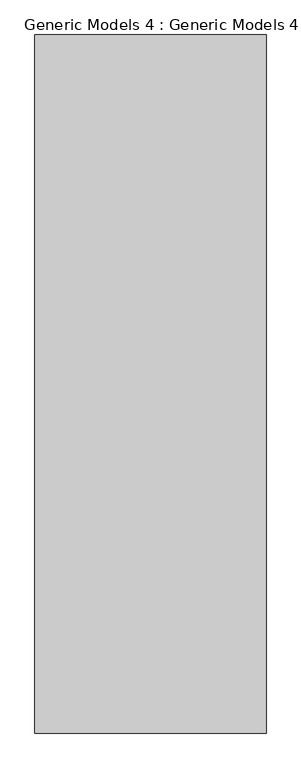
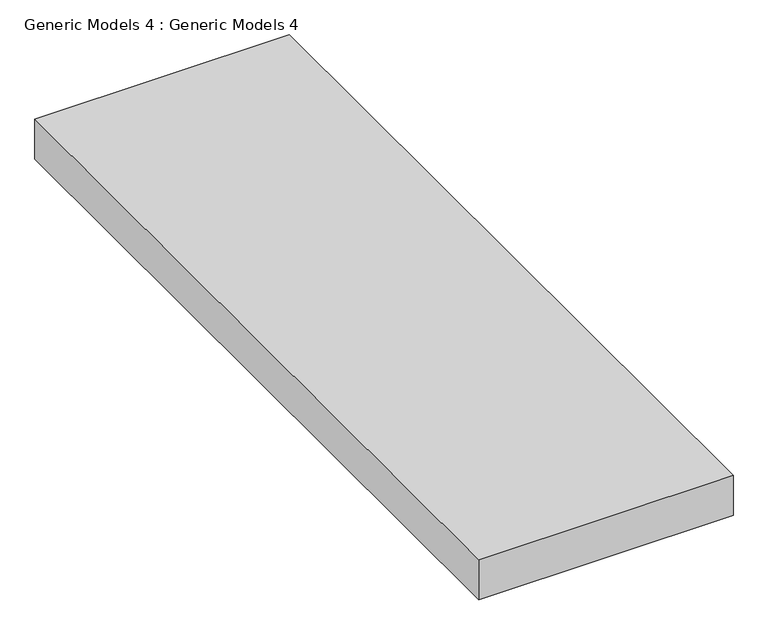
"""IFC4 building model written with IfcOpenShell, lengths in millimetres: proxy geometry, Generic Models 4 : Generic Models 4."""

from ifc_helpers import new_model, si_unit, frame, origin, place, context, project, spatial, polyline, outline, extrude, source, transform, mapped, element, save


def generic_models_4_generic_models_4_668f170e(model_context):
    return source(origin(), model_context, "Body", "SweptSolid", [
        extrude(outline(polyline([(-42988.0145004, 5090.4756148), (-42988.0145004, 7852.6472085), (-42073.6145004, 7852.6472085), (-42073.6145004, 5090.4756148), (-42988.0145004, 5090.4756148)])), frame((0.0, 0.0, 2800.3772468), z_axis=(0.0, 0.0, 1.0), x_axis=(1.0, 0.0, 0.0)), (0.0, 0.0, 1.0), 152.4),
    ])


if __name__ == "__main__":
    model = new_model("IFC4")
    model_context = context("Model", 3, world=origin())
    ifc_project = project(units=[si_unit("LENGTHUNIT", "METRE", prefix="MILLI")], contexts=[model_context])
    site = spatial("IfcSite", under=ifc_project)
    building = spatial("IfcBuilding", under=site)
    placement = place(None, origin())
    generic_models_4_generic_models_4_shape = generic_models_4_generic_models_4_668f170e(model_context)
    element("IfcBuildingElementProxy", 1, Name="Generic Models 4 : Generic Models 4", ObjectType="Generic Models 4 : Generic Models 4", at=placement, inside=building, context=model_context, shape_type="MappedRepresentation", body=[
        mapped(generic_models_4_generic_models_4_shape, transform((0.0, 0.0, 0.0), x_axis=(1.0, 0.0, 0.0), y_axis=(0.0, 1.0, 0.0), z_axis=(0.0, 0.0, 1.0))),
    ])
    save(model, "model.ifc")
